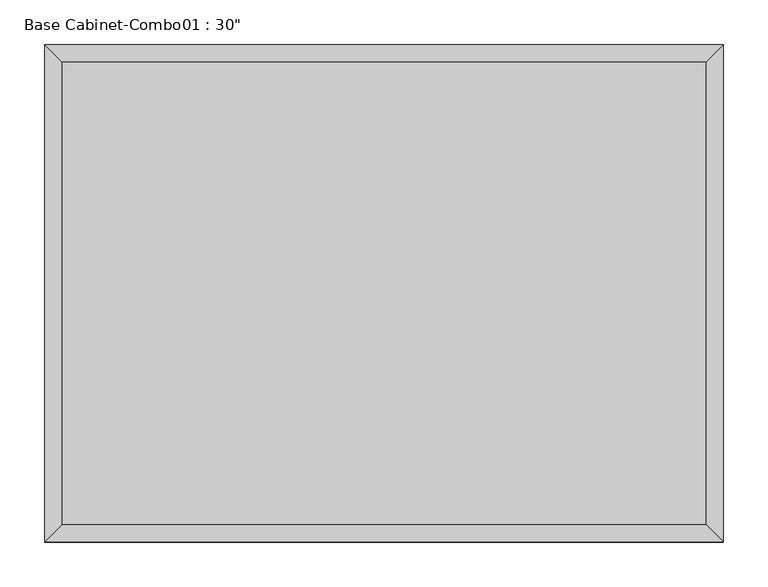
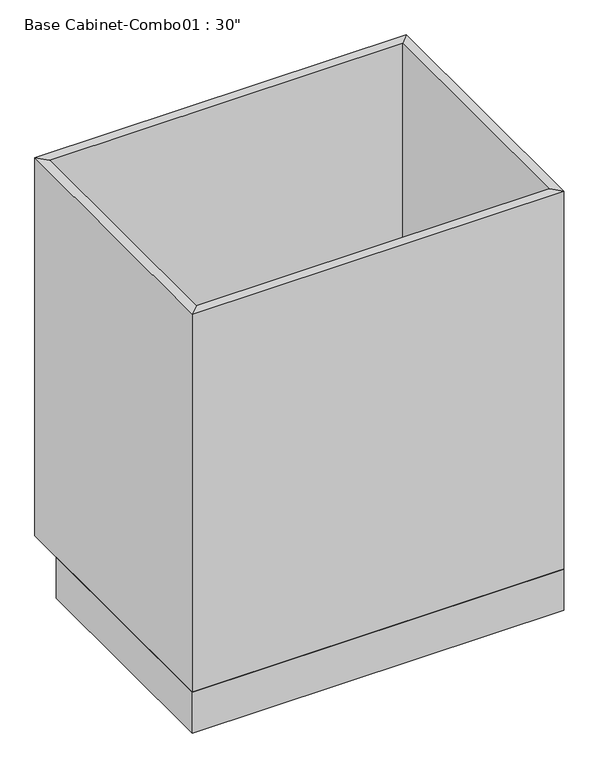
"""IFC4 building model written with IfcOpenShell, lengths in millimetres: furniture geometry."""

from ifc_helpers import new_model, si_unit, frame, origin, origin_with_axes, place, context, project, spatial, polyline, outline, extrude, faceted_brep, source, transform, mapped, element, save


def furniture_a56de0b1(model_context):
    return source(origin(), model_context, "Body", "SolidModel", [
        extrude(outline(polyline([(399.7377049, 0.0), (-362.2622951, 0.0), (-362.2622951, 482.6), (399.7377049, 482.6), (399.7377049, 0.0)])), origin_with_axes(), (0.0, 0.0, 1.0), 88.9),
        faceted_brep([(380.6877049, 539.75, 908.05), (-343.2122951, 539.75, 908.05), (-343.2122951, 539.75, 88.9), (380.6877049, 539.75, 88.9), (399.7377049, 558.8, 908.05), (-362.2622951, 558.8, 908.05), (399.7377049, 558.8, 88.9), (-362.2622951, 558.8, 88.9), (-343.2122951, 19.05, 908.05), (-343.2122951, 19.05, 88.9), (-362.2622951, 0.0, 908.05), (-362.2622951, 0.0, 88.9), (380.6877049, 19.05, 908.05), (380.6877049, 19.05, 88.9), (399.7377049, 0.0, 908.05), (399.7377049, 0.0, 88.9)], [[[0, 1, 2, 3]], [[4, 5, 1, 0]], [[6, 7, 5, 4]], [[3, 2, 7, 6]], [[1, 8, 9, 2]], [[5, 10, 8, 1]], [[7, 11, 10, 5]], [[2, 9, 11, 7]], [[8, 12, 13, 9]], [[10, 14, 12, 8]], [[11, 15, 14, 10]], [[9, 13, 15, 11]], [[12, 0, 3, 13]], [[14, 4, 0, 12]], [[15, 6, 4, 14]], [[13, 3, 6, 15]]]),
        extrude(outline(polyline([(380.6877049, 19.05), (-343.2122951, 19.05), (-343.2122951, 539.75), (380.6877049, 539.75), (380.6877049, 19.05)])), frame((0.0, 0.0, 88.9), z_axis=(0.0, 0.0, 1.0), x_axis=(1.0, 0.0, 0.0)), (0.0, 0.0, 1.0), 19.05),
    ])


if __name__ == "__main__":
    model = new_model("IFC4")
    model_context = context("Model", 3, world=origin())
    ifc_project = project(units=[si_unit("LENGTHUNIT", "METRE", prefix="MILLI")], contexts=[model_context])
    site = spatial("IfcSite", under=ifc_project)
    building = spatial("IfcBuilding", under=site)
    placement = place(None, origin())
    furniture_shape = furniture_a56de0b1(model_context)
    element("IfcFurniture", 1, ObjectType="Base Cabinet-Combo01 : 30\"", at=placement, inside=building, context=model_context, shape_type="MappedRepresentation", body=[
        mapped(furniture_shape, transform((0.0, 0.0, 0.0), x_axis=(1.0, 0.0, 0.0), y_axis=(0.0, 1.0, 0.0), z_axis=(0.0, 0.0, 1.0))),
    ])
    save(model, "model.ifc")

# Revit data of these elements
# Type "Base Cabinet-Combo01 : 30\""
#   Depth = 1' - 10"
#   Height = 2' - 11 3/4"
#   Toe Depth = 0' - 3"
#   Toe Height = 0' - 3 1/2"
#   Width = 2' - 6"
#   Default Elevation = 0
# Element 1 (IfcFurniture, "Base Cabinet-Combo01 : 30\"")
#   Materials on its faces: "Cabinet"
# Materials
#   "Cabinet": colour RGB 204 122 2, transparency 0
